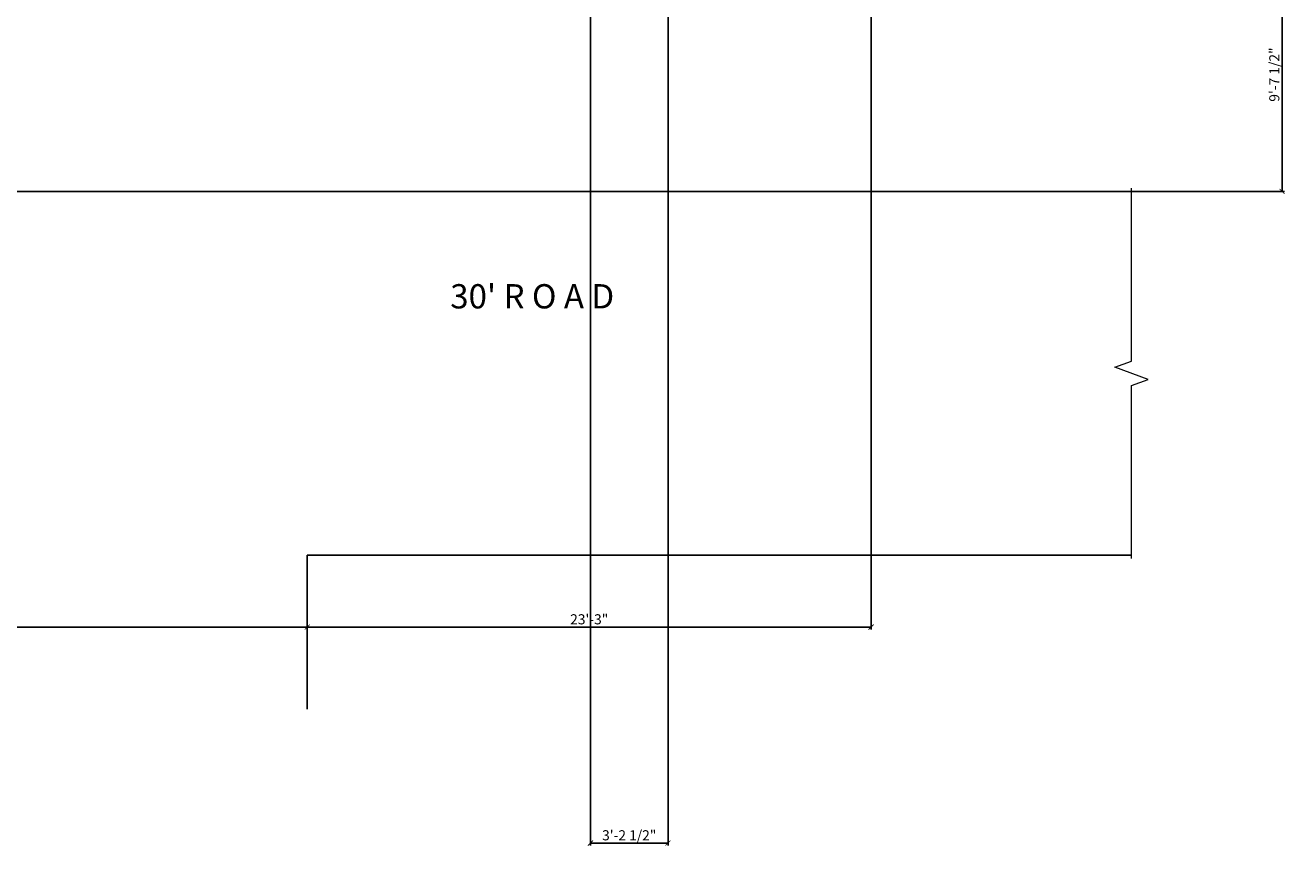
# Model space of a CAD drawing. Units: inches. Extents: x 3283068 to 3284536, y 3240756 to 3241803.
# Tile 17 of 19: x 3283910 to 3284536, y 3240756 to 3241165. Entities that reach past the tile are written whole.
import ezdxf

# ---------------------------------------------------------------- set-up
doc = ezdxf.new("R2010")
doc.units = ezdxf.units.IN
for name, color, linetype, lineweight in [('A-ANNO-DIMS', 2, 'Continuous', 18), ('C-ANNO-SYMB', 7, 'Continuous', 18), ('C-ANNO-TEXT', 7, 'Continuous', 18), ('C-PROP', 7, 'Continuous', 25), ('C-ROAD', 8, 'Continuous', 25)]:
    doc.layers.add(name, color=color, linetype=linetype, lineweight=lineweight)
doc.styles.get("Standard").update_dxf_attribs({"font": 'arial.ttf'})
doc.dimstyles.new('ISO-25', dxfattribs={"dimtxt": 5, "dimasz": 2.5, "dimexe": 1.25, "dimexo": 0.625, "dimtad": 1, "dimlunit": 4, "dimtxsty": 'Standard', "dimblk": 'ARCHTICK', "dimcen": 2.5, "dimadec": 0, "dimazin": 0, "dimtfac": 1, "dimtmove": 0, "dimatfit": 3, "dimfxl": 1, "dimarcsym": 0})

# ---------------------------------------------------------------- blocks, each defined once
blk = doc.blocks.new('_ArchTick')
at = {"color": 0, "linetype": 'ByBlock', "const_width": 0.15}
blk.add_lwpolyline([(-0.5, -0.5), (0.5, 0.5)], dxfattribs=at)
blk = doc.blocks.new('*D32')
at = {"layer": 'A-ANNO-DIMS', "color": 0, "lineweight": -2, "transparency": 16777216}
for p, q in [((3283572.09, 3240901.98), (3283572.09, 3240865.87)), ((3283572.09, 3240867.12), (3284049.09, 3240867.12)), ((3284049.09, 3240867.75), (3284049.09, 3240868.37))]:
    blk.add_line(p, q, dxfattribs=at)
at = {"layer": 'Defpoints', "color": 0, "transparency": 16777216}
for p in [(3283572.09, 3240902.6), (3284049.09, 3240867.12), (3284049.09, 3240867.12)]:
    blk.add_point(p, dxfattribs=at)
at = {"layer": 'A-ANNO-DIMS', "color": 0, "lineweight": -2, "transparency": 16777216, "xscale": 2.5, "yscale": 2.5, "zscale": 2.5, "rotation": 180}
blk.add_blockref('_ArchTick', (3283572.09, 3240867.12), dxfattribs=at)
at = {"layer": 'A-ANNO-DIMS', "color": 0, "lineweight": -2, "transparency": 16777216, "xscale": 2.5, "yscale": 2.5, "zscale": 2.5}
blk.add_blockref('_ArchTick', (3284049.09, 3240867.12), dxfattribs=at)
at = {"layer": 'A-ANNO-DIMS', "color": 0, "transparency": 16777216, "insert": (3283810.59, 3240870.3), "char_height": 5, "attachment_point": 5}
blk.add_mtext('39\'-9"', dxfattribs=at)
blk = doc.blocks.new('*D33')
at = {"layer": 'A-ANNO-DIMS', "color": 0, "lineweight": -2, "transparency": 16777216}
for p, q in [((3284328.09, 3241081.98), (3284328.09, 3240865.87)), ((3284049.09, 3240867.75), (3284049.09, 3240868.37)), ((3284049.09, 3240867.12), (3284328.09, 3240867.12))]:
    blk.add_line(p, q, dxfattribs=at)
at = {"layer": 'Defpoints', "color": 0, "transparency": 16777216}
for p in [(3284328.09, 3241082.6), (3284049.09, 3240867.12), (3284328.09, 3240867.12)]:
    blk.add_point(p, dxfattribs=at)
at = {"layer": 'A-ANNO-DIMS', "color": 0, "lineweight": -2, "transparency": 16777216, "xscale": 2.5, "yscale": 2.5, "zscale": 2.5, "rotation": 180}
blk.add_blockref('_ArchTick', (3284049.09, 3240867.12), dxfattribs=at)
at = {"layer": 'A-ANNO-DIMS', "color": 0, "lineweight": -2, "transparency": 16777216, "xscale": 2.5, "yscale": 2.5, "zscale": 2.5}
blk.add_blockref('_ArchTick', (3284328.09, 3240867.12), dxfattribs=at)
at = {"layer": 'A-ANNO-DIMS', "color": 0, "transparency": 16777216, "insert": (3284188.59, 3240870.3), "char_height": 5, "attachment_point": 5}
blk.add_mtext('23\'-3"', dxfattribs=at)
blk = doc.blocks.new('ROAD-BREAK')
blk.add_lwpolyline([(8.24, 0), (8.24, 85.5), (16.48, 88.5), (0, 94.5), (8.24, 97.5), (8.24, 183)])
blk = doc.blocks.new('*D62')
at = {"layer": 'A-ANNO-DIMS', "color": 0, "lineweight": -2, "transparency": 16777216}
for p, q in [((3284237.21, 3241198.1), (3284532.74, 3241198.1)), ((3284531.49, 3241198.1), (3284531.49, 3241082.6)), ((3284328.71, 3241082.6), (3284532.74, 3241082.6))]:
    blk.add_line(p, q, dxfattribs=at)
at = {"layer": 'Defpoints', "color": 0, "transparency": 16777216}
for p in [(3284236.59, 3241198.1), (3284328.09, 3241082.6), (3284531.49, 3241082.6)]:
    blk.add_point(p, dxfattribs=at)
at = {"layer": 'A-ANNO-DIMS', "color": 0, "lineweight": -2, "transparency": 16777216, "xscale": 2.5, "yscale": 2.5, "zscale": 2.5}
for p, rotation in [((3284531.49, 3241198.1), 90), ((3284531.49, 3241082.6), 270)]:
    blk.add_blockref('_ArchTick', p, dxfattribs=dict(at, rotation=rotation))
at = {"layer": 'A-ANNO-DIMS', "color": 0, "transparency": 16777216, "insert": (3284528.28, 3241140.35), "char_height": 5, "attachment_point": 5, "rotation": 90}
blk.add_mtext('9\'-7 1/2"', dxfattribs=at)
blk = doc.blocks.new('*D63')
at = {"layer": 'A-ANNO-DIMS', "color": 0, "lineweight": -2, "transparency": 16777216}
for p, q in [((3283248.09, 3241083.23), (3283248.09, 3241798.08)), ((3283248.09, 3241796.83), (3284328.09, 3241796.83)), ((3284328.09, 3241083.23), (3284328.09, 3241798.08))]:
    blk.add_line(p, q, dxfattribs=at)
at = {"layer": 'Defpoints', "color": 0, "transparency": 16777216}
for p in [(3284328.09, 3241796.83), (3283248.09, 3241082.6), (3284328.09, 3241082.6)]:
    blk.add_point(p, dxfattribs=at)
at = {"layer": 'A-ANNO-DIMS', "color": 0, "lineweight": -2, "transparency": 16777216, "xscale": 2.5, "yscale": 2.5, "zscale": 2.5, "rotation": 180}
blk.add_blockref('_ArchTick', (3283248.09, 3241796.83), dxfattribs=at)
at = {"layer": 'A-ANNO-DIMS', "color": 0, "lineweight": -2, "transparency": 16777216, "xscale": 2.5, "yscale": 2.5, "zscale": 2.5}
blk.add_blockref('_ArchTick', (3284328.09, 3241796.83), dxfattribs=at)
at = {"layer": 'A-ANNO-DIMS', "color": 0, "transparency": 16777216, "insert": (3283788.09, 3241800.01), "char_height": 5, "attachment_point": 5}
blk.add_mtext('90\'-0"', dxfattribs=at)
blk = doc.blocks.new('*D65')
at = {"layer": 'A-ANNO-DIMS', "color": 0, "lineweight": -2, "transparency": 16777216}
for p, q in [((3284189.18, 3241264.98), (3284189.18, 3240759.03)), ((3284227.59, 3241264.98), (3284227.59, 3240759.03)), ((3284189.18, 3240760.28), (3284227.59, 3240760.28))]:
    blk.add_line(p, q, dxfattribs=at)
at = {"layer": 'Defpoints', "color": 0, "transparency": 16777216}
for p in [(3284189.18, 3241265.6), (3284227.59, 3241265.6), (3284227.59, 3240760.28)]:
    blk.add_point(p, dxfattribs=at)
at = {"layer": 'A-ANNO-DIMS', "color": 0, "lineweight": -2, "transparency": 16777216, "xscale": 2.5, "yscale": 2.5, "zscale": 2.5, "rotation": 180}
blk.add_blockref('_ArchTick', (3284189.18, 3240760.28), dxfattribs=at)
at = {"layer": 'A-ANNO-DIMS', "color": 0, "lineweight": -2, "transparency": 16777216, "xscale": 2.5, "yscale": 2.5, "zscale": 2.5}
blk.add_blockref('_ArchTick', (3284227.59, 3240760.28), dxfattribs=at)
at = {"layer": 'A-ANNO-DIMS', "color": 0, "transparency": 16777216, "insert": (3284208.39, 3240763.49), "char_height": 5, "attachment_point": 5}
blk.add_mtext('3\'-2 1/2"', dxfattribs=at)

msp = doc.modelspace()

# ---------------------------------------------------------------- linework, layer by layer
at = {"layer": 'C-PROP'}
for p in [(3284328.089, 3241730.602), (3283248.089, 3241082.602)]:
    msp.add_line(p, (3284328.089, 3241082.602), dxfattribs=at)
at = {"layer": 'C-ROAD'}
for p, q in [((3284328.089, 3241082.602), (3284457.021, 3241082.602)), ((3284457.021, 3240902.602), (3284049.089, 3240902.602)), ((3284049.089, 3240902.602), (3284049.089, 3240826.506)), ((3284049.089, 3240902.602), (3284328.089, 3240902.602))]:
    msp.add_line(p, q, dxfattribs=at)

# ---------------------------------------------------------------- block references
at = {"layer": 'C-ANNO-SYMB'}
msp.add_blockref('ROAD-BREAK', (3284448.779, 3240901.102), dxfattribs=at)

# ---------------------------------------------------------------- texts
at = {"layer": 'C-ANNO-TEXT', "insert": (3284119.804, 3241036.697), "char_height": 12, "attachment_point": 1}
msp.add_mtext_dynamic_manual_height_columns("30' R O A D", width=123.55873, gutter_width=12.5, heights=[0], dxfattribs=at)

# ---------------------------------------------------------------- dimensions: what is measured, and where the dimension line sits
at = {"layer": 'A-ANNO-DIMS'}
for base, p1, p2, override, picture, middle in [((3284328.089, 3241796.827), (3283248.089, 3241082.602), (3284328.089, 3241082.602), {"dimdec": 1, "dimlfac": 1, "dimrnd": 0, "dimzin": 1, "dimdsep": 46, "dimlunit": 4, "dimfrac": 2}, '*D63', (3283788.089, 3241800.005)), ((3284227.589, 3240760.281), (3284189.185, 3241265.602), (3284227.589, 3241265.602), {"dimdec": 1, "dimlfac": 1, "dimrnd": 0, "dimzin": 1, "dimdsep": 46, "dimlunit": 4, "dimfrac": 2}, '*D65', (3284208.387, 3240763.493)), ((3284328.089, 3240867.124), (3284049.089, 3240867.124), (3284328.089, 3241082.602), {"dimclrd": 0, "dimclre": 0, "dimclrt": 0, "dimtmove": 1}, '*D33', (3284188.589, 3240870.304)), ((3284049.089, 3240867.124), (3283572.089, 3240902.602), (3284049.089, 3240867.124), {"dimclrd": 0, "dimclre": 0, "dimclrt": 0, "dimtmove": 1}, '*D32', (3283810.589, 3240870.304))]:
    dim = msp.add_linear_dim(base=base, p1=p1, p2=p2, dimstyle='ISO-25', override=override, dxfattribs=at)
    dim.commit()
    dim.dimension.update_dxf_attribs({"geometry": picture, "text_midpoint": middle})
dim = msp.add_linear_dim(base=(3284531.489, 3241082.602), p1=(3284236.589, 3241198.102), p2=(3284328.089, 3241082.602), angle=90, dimstyle='ISO-25', override={"dimdec": 1, "dimlfac": 1, "dimrnd": 0, "dimzin": 1, "dimdsep": 46, "dimlunit": 4, "dimfrac": 2}, dxfattribs=at)
dim.commit()
dim.dimension.update_dxf_attribs({"geometry": '*D62', "text_midpoint": (3284528.278, 3241140.352)})

doc.saveas('drawing.dxf')
